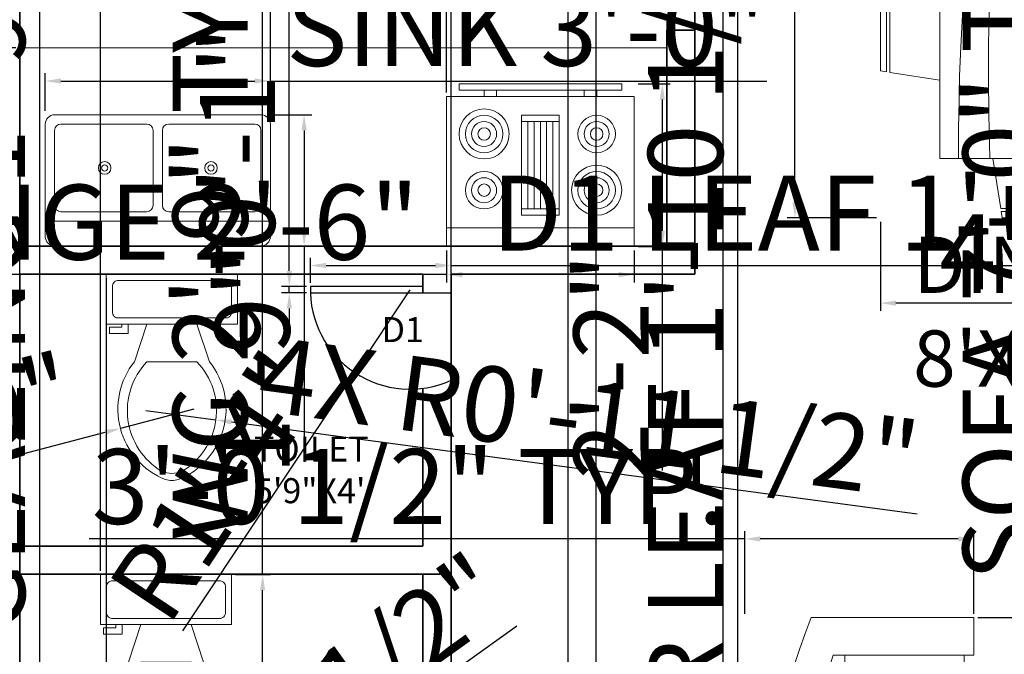
# Model space of a CAD drawing. Units: inches. Extents: x 2691 to 3133, y 1294 to 1993.
# Tile 4 of 7: x 2777 to 2935, y 1696 to 1798. Entities that reach past the tile are written whole.
import ezdxf

# ---------------------------------------------------------------- set-up
doc = ezdxf.new("R2010")
doc.units = ezdxf.units.IN
for name, color, linetype, lineweight in [('A-ANNO-DIMS', 2, 'Continuous', 18), ('A-ANNO-TEXT', 7, 'Continuous', 18), ('A-AREA-IDEN', 7, 'Continuous', 25), ('A-DOOR', 3, 'Continuous', 25), ('A-EQPM', 8, 'Continuous', 18), ('A-FLOR-FIXT', 9, 'Continuous', 18), ('A-FURN', 8, 'Continuous', 18), ('A-WALL', 7, 'Continuous', 35)]:
    doc.layers.add(name, color=color, linetype=linetype, lineweight=lineweight)
doc.styles.get("Standard").update_dxf_attribs({"font": 'arial.ttf'})
doc.dimstyles.new('ISO-25', dxfattribs={"dimtxt": 12, "dimasz": 2.5, "dimexe": 1.25, "dimexo": 0.625, "dimtad": 1, "dimdec": 1, "dimlunit": 3, "dimtxsty": 'Standard', "dimcen": 2.5, "dimadec": 0, "dimazin": 0, "dimtfac": 1, "dimtdec": 1, "dimtmove": 0, "dimatfit": 3, "dimfxl": 1, "dimarcsym": 0})

# ---------------------------------------------------------------- blocks, each defined once
blk = doc.blocks.new('Sofa - Roundback 7 ft.')
for p, q in [((-12.00002, -32.4421), (-12.00003, -6.5971)), ((11.99997, -32.4421), (11.99998, -6.5971)), ((-36.000027, -34), (-36.000027, -11.4696)), ((35.99998, -34), (35.99998, -11.4696)), ((-35.999844, -13.3819), (35.9998, -13.3819)), ((-36.000027, -32.4421), (35.99998, -32.4421))]:
    blk.add_line(p, q)
for points in [[(-36.000027, -34), (-42.000027, -34), (-42.000027, -8)], [(41.99998, -8), (41.99998, -34), (35.99998, -34)]]:
    blk.add_lwpolyline(points)
for centre, radius, start, end in [((0, -114.25), 114.25, 68.43141, 111.5686), ((-0.00001, -127.1968), 121.1968, 72.72033, 107.2797)]:
    blk.add_arc(centre, radius, start, end)
blk = doc.blocks.new('Dining Set - 36 x 72 in.')
for p, q in [((-22, 27.5), (-22.1562, 26.50042)), ((-22, 27.5), (-6, 27.5)), ((-5.8437, 26.49966), (-6, 27.5)), ((6, 27.5), (5.8438, 26.50042)), ((6, 27.5), (22, 27.5)), ((22.1563, 26.49966), (22, 27.5)), ((-22.2343, 26.00059), (-23.4847, 17.99762)), ((-22.2304, 26), (-5.7608, 26)), ((-5.8416, 26.5), (-22.1534, 26.5)), ((-4.5152, 17.99762), (-5.7655, 25.99926)), ((5.7657, 26.00059), (4.5153, 17.99762)), ((5.7696, 26), (22.2392, 26)), ((22.1584, 26.5), (5.8466, 26.5)), ((23.4848, 17.99762), (22.2345, 25.99926)), ((36, 18), (-36, 18)), ((-36, 18), (-36, -18)), ((36, -18), (36, 18)), ((-44.0006, 8.23428), (-35.9976, 9.48474)), ((44.0006, 8.23428), (35.9976, 9.48474)), ((-45.5, 8), (-44.5004, 8.15617)), ((-45.5, 8), (-45.5, -8)), ((-44.5, -8.15843), (-44.5, 8.15338)), ((-44, 8.23041), (-44, -8.23915)), ((44, 8.23041), (44, -8.23915)), ((44.5, -8.15843), (44.5, 8.15338)), ((45.5, 8), (44.5005, 8.15617)), ((45.5, 8), (45.5, -8)), ((-44.4997, -8.15631), (-45.5, -8)), ((-35.9976, -9.48476), (-43.9993, -8.2345)), ((35.9976, -9.48476), (43.9993, -8.2345)), ((44.4997, -8.15631), (45.5, -8)), ((-36, -18), (36, -18)), ((-22.2343, -26.0006), (-23.4847, -17.99762)), ((-4.5152, -17.99762), (-5.7655, -25.99928)), ((5.7657, -26.0006), (4.5153, -17.99762)), ((23.4848, -17.99762), (22.2345, -25.99928)), ((-22.2304, -26), (-5.7608, -26)), ((-22, -27.5), (-22.1562, -26.50044)), ((-5.8416, -26.5), (-22.1534, -26.5)), ((-5.8437, -26.49967), (-6, -27.5)), ((5.7696, -26), (22.2392, -26)), ((6, -27.5), (5.8438, -26.50044)), ((22.1584, -26.5), (5.8466, -26.5)), ((22.1563, -26.49967), (22, -27.5)), ((-22, -27.5), (-6, -27.5)), ((6, -27.5), (22, -27.5))]:
    blk.add_line(p, q)
for points in [[(-36, 15), (-31.1772, 14.97754), (-26.8079, 14.91406), (-22.8538, 14.81543), (-19.276, 14.6875), (-16.0362, 14.53613), (-13.0957, 14.36718), (-10.4159, 14.18652), (-7.9583, 14), (-5.6904, 13.81315), (-3.6035, 13.63021), (-1.6954, 13.45508), (0.0365, 13.29166), (1.5945, 13.14388), (2.9811, 13.01562), (4.1988, 12.9108), (5.25, 12.83333), (6.1393, 12.78613), (6.8802, 12.76823), (7.4883, 12.77767), (7.9792, 12.8125), (8.3685, 12.87077), (8.6719, 12.95052), (8.9049, 13.0498), (9.0833, 13.16666), (9.2205, 13.29899), (9.3216, 13.44401), (9.3895, 13.59879), (9.4271, 13.76041), (9.4373, 13.92594), (9.4232, 14.09245), (9.3875, 14.257), (9.3333, 14.41666), (9.2638, 14.56917), (9.1836, 14.71484), (9.0975, 14.85465), (9.0104, 14.98958), (8.9272, 15.1206), (8.8529, 15.2487), (8.7922, 15.37483), (8.75, 15.5), (8.7305, 15.62467), (8.7344, 15.74739), (8.7617, 15.86621), (8.8125, 15.97916), (8.8867, 16.08431), (8.9844, 16.17968), (9.1055, 16.26334), (9.25, 16.33333), (9.4189, 16.38802), (9.6172, 16.42708), (9.8506, 16.45052), (10.125, 16.45833), (10.4463, 16.45052), (10.8203, 16.42708), (11.2529, 16.38802), (11.75, 16.33333), (12.3184, 16.26318), (12.9694, 16.17838), (13.7151, 16.07991), (14.5677, 15.96875), (15.5395, 15.84586), (16.6426, 15.71224), (17.8893, 15.56884), (19.2917, 15.41666), (20.859, 15.25667), (22.5879, 15.08984), (24.4721, 14.91715), (26.5052, 14.73958), (28.6809, 14.5581), (30.9929, 14.3737), (33.4347, 14.18733), (36, 14)], [(-36, 10), (-28.9766, 10.14274), (-23.1725, 10.20442), (-18.4241, 10.19775), (-14.5677, 10.13541), (-11.4399, 10.03011), (-8.877, 9.89453), (-6.7154, 9.74137), (-4.7917, 9.58333), (-2.9698, 9.43082), (-1.2246, 9.28515), (0.4415, 9.14534), (2.026, 9.01041), (3.5266, 8.87939), (4.9408, 8.7513), (6.266, 8.62516), (7.5, 8.5), (8.6411, 8.37549), (9.6914, 8.2539), (10.6538, 8.13818), (11.5312, 8.03125), (12.3267, 7.93603), (13.043, 7.85547), (13.6831, 7.79248), (14.25, 7.75), (14.7471, 7.7303), (15.1797, 7.73307), (15.5537, 7.75732), (15.875, 7.80208), (16.1494, 7.86637), (16.3828, 7.94922), (16.5811, 8.04964), (16.75, 8.16666), (16.8944, 8.29915), (17.0143, 8.44531), (17.1089, 8.60319), (17.1771, 8.77083), (17.218, 8.94629), (17.2305, 9.1276), (17.2137, 9.31282), (17.1667, 9.5), (17.0895, 9.6875), (16.987, 9.875), (16.8649, 10.0625), (16.7292, 10.25), (16.5856, 10.4375), (16.4401, 10.625), (16.2985, 10.8125), (16.1667, 11), (16.05, 11.18733), (15.9518, 11.3737), (15.8752, 11.5581), (15.8229, 11.73958), (15.798, 11.91715), (15.8034, 12.08984), (15.842, 12.25667), (15.9167, 12.41666), (16.0295, 12.56836), (16.1784, 12.70833), (16.3605, 12.83268), (16.5729, 12.9375), (16.8127, 13.01888), (17.0768, 13.07291), (17.3625, 13.0957), (17.6667, 13.08333), (17.9894, 13.03312), (18.3418, 12.94726), (18.7382, 12.82918), (19.1927, 12.68229), (19.7195, 12.51001), (20.3327, 12.31575), (21.0465, 12.10294), (21.875, 11.875), (22.8357, 11.63354), (23.959, 11.37304), (25.2786, 11.08618), (26.8282, 10.76562), (28.6414, 10.40405), (30.752, 9.99414), (33.1936, 9.52856), (36, 9)], [(-36, 5.5), (-30.7157, 5.3348), (-26.069, 5.20963), (-21.9946, 5.11767), (-18.4271, 5.05208), (-15.3009, 5.00602), (-12.5508, 4.97265), (-10.1112, 4.94515), (-7.9167, 4.91666), (-5.909, 4.88167), (-4.0586, 4.83984), (-2.3429, 4.79215), (-0.7396, 4.73958), (0.7739, 4.6831), (2.22, 4.6237), (3.6213, 4.56233), (5, 4.5), (6.373, 4.43782), (7.7344, 4.3776), (9.0723, 4.32129), (10.375, 4.27083), (11.6309, 4.22819), (12.8281, 4.19531), (13.9551, 4.17415), (15, 4.16666), (15.954, 4.17448), (16.819, 4.19791), (17.6001, 4.23698), (18.3021, 4.29166), (18.9299, 4.36198), (19.4883, 4.44791), (19.9823, 4.54948), (20.4167, 4.66666), (20.7969, 4.79899), (21.1302, 4.94401), (21.4245, 5.09879), (21.6875, 5.26041), (21.9271, 5.42594), (22.1511, 5.59245), (22.3672, 5.757), (22.5834, 5.91666), (22.8065, 6.06868), (23.0404, 6.21093), (23.2879, 6.34147), (23.5521, 6.45833), (23.8358, 6.55957), (24.142, 6.64323), (24.4735, 6.70735), (24.8334, 6.75), (25.2235, 6.76969), (25.642, 6.76692), (26.0858, 6.74267), (26.5521, 6.69791), (27.0379, 6.63362), (27.5404, 6.55078), (28.0565, 6.45036), (28.5834, 6.33333), (29.1242, 6.19987), (29.7071, 6.04687), (30.3661, 5.87044), (31.1354, 5.66666), (32.0493, 5.43164), (33.142, 5.16146), (34.4475, 4.85221), (36, 4.5)], [(-36, -1), (-30.7915, -0.6591), (-26.0195, -0.38216), (-21.6519, -0.16284), (-17.6563, 0.00521), (-14.0005, 0.12833), (-10.6523, 0.21289), (-7.5796, 0.26522), (-4.75, 0.29166), (-2.134, 0.29793), (0.2878, 0.28711), (2.5317, 0.26163), (4.6146, 0.22396), (6.5529, 0.17651), (8.3633, 0.12174), (10.0623, 0.06209), (11.6667, 0), (13.1899, -0.06201), (14.6341, -0.1211), (15.9982, -0.17432), (17.2813, -0.21875), (18.4823, -0.25147), (19.6003, -0.26953), (20.6343, -0.27002), (21.5834, -0.25), (22.4481, -0.20768), (23.2357, -0.14584), (23.9549, -0.06836), (24.6146, 0.02083), (25.2235, 0.11784), (25.7904, 0.21875), (26.3241, 0.31966), (26.8334, 0.41666), (27.3265, 0.50618), (27.8099, 0.58593), (28.2894, 0.65397), (28.7709, 0.70833), (29.2601, 0.74707), (29.763, 0.76823), (30.2855, 0.76985), (30.8334, 0.75), (31.4088, 0.70784), (31.9994, 0.64713), (32.589, 0.57275), (33.1615, 0.48958), (33.7008, 0.4025), (34.1908, 0.3164), (34.6153, 0.23616), (34.9584, 0.16666), (35.2099, 0.11165), (35.3848, 0.07031), (35.504, 0.04069), (35.5886, 0.02083), (35.6594, 0.00879), (35.7377, 0.0026), (35.8442, 0.00032), (36, 0)], [(-36, -6.5), (-27.1843, -6.31267), (-20.084, -6.1263), (-14.469, -5.9419), (-10.1094, -5.76042), (-6.7752, -5.58285), (-4.2363, -5.41016), (-2.2629, -5.24333), (-0.625, -5.08334), (0.8708, -4.93099), (2.2715, -4.78646), (3.5872, -4.64974), (4.8281, -4.52084), (6.0046, -4.39974), (7.127, -4.28646), (8.2053, -4.18099), (9.25, -4.08334), (10.2705, -3.99382), (11.2734, -3.91407), (12.2647, -3.84603), (13.25, -3.79167), (14.2354, -3.75293), (15.2266, -3.73177), (16.2295, -3.73015), (17.25, -3.75), (18.2912, -3.79248), (19.3451, -3.85547), (20.4009, -3.93604), (21.4479, -4.03125), (22.4754, -4.13819), (23.4727, -4.25391), (24.4289, -4.37549), (25.3334, -4.5), (26.1785, -4.62492), (26.9694, -4.74935), (27.7145, -4.87281), (28.4219, -4.99479), (29.1, -5.11483), (29.7572, -5.23242), (30.4016, -5.34709), (31.0417, -5.45834), (31.6837, -5.56437), (32.3262, -5.65821), (32.9658, -5.73153), (33.599, -5.77604), (34.2224, -5.78345), (34.8327, -5.74545), (35.4264, -5.65373), (36, -5.5)], [(-36, -10), (-26.4022, -9.81299), (-18.4675, -9.62891), (-11.9839, -9.45069), (-6.7396, -9.28125), (-2.5226, -9.12354), (0.8789, -8.98047), (3.6769, -8.85498), (6.0833, -8.75), (8.2767, -8.66765), (10.3021, -8.60677), (12.1712, -8.56543), (13.8958, -8.54167), (15.4876, -8.53353), (16.9583, -8.53907), (18.3197, -8.55632), (19.5834, -8.58334), (20.7616, -8.61841), (21.8685, -8.66081), (22.9188, -8.71004), (23.9271, -8.76563), (24.9081, -8.82707), (25.8763, -8.89388), (26.8465, -8.96558), (27.8334, -9.04167), (28.8474, -9.12118), (29.8828, -9.20117), (30.93, -9.27824), (31.9792, -9.34896), (33.0205, -9.40991), (34.0443, -9.45768), (35.0407, -9.48885), (36, -9.5)], [(-36, -14.5), (-30.0881, -14.33513), (-25.0332, -14.21224), (-20.7312, -14.12647), (-17.0781, -14.07292), (-13.97, -14.04671), (-11.3027, -14.04297), (-8.9724, -14.05681), (-6.875, -14.08334), (-4.9224, -14.11833), (-3.0905, -14.16016), (-1.3709, -14.20785), (0.2448, -14.26042), (1.7647, -14.3169), (3.1973, -14.3763), (4.5507, -14.43767), (5.8333, -14.5), (7.0554, -14.5621), (8.235, -14.62175), (9.3922, -14.67652), (10.5469, -14.72396), (11.7192, -14.76164), (12.929, -14.78711), (14.1965, -14.79794), (15.5417, -14.79167), (16.9933, -14.76424), (18.6152, -14.70508), (20.4804, -14.60197), (22.6615, -14.44271), (25.2312, -14.21509), (28.2624, -13.9069), (31.8277, -13.50594), (36, -13)]]:
    blk.add_lwpolyline(points)
blk = doc.blocks.new('Toilet - top')
for p, q in [((9.5, -6), (9.5, -2)), ((-10, -8.5), (-8, -8.5)), ((-10, -9.5), (-10, -8.5)), ((-8, -8.5), (-8, -8)), ((-7, -8), (-7, -9.5)), ((-4, -8), (-6, -14)), ((4, -8), (6, -14)), ((-7, -9.5), (-10, -9.5)), ((4, -14), (-4, -14))]:
    blk.add_line(p, q)
blk.add_lwpolyline([(10.5, -8), (10.5, 0), (-10.5, 0), (-10.5, -8)], close=True)
for points in [[(8.5, -1), (-8.5, -1)], [(-9.5, -2), (-9.5, -6)], [(-8.5, -7), (8.5, -7)]]:
    blk.add_lwpolyline(points)
for centre, radius, start, end in [((-8.62, -1.88), 0.884, 81.8699, 188.1301), ((8.62, -1.88), 0.884, 351.8699, 98.1301), ((-8.62, -6.12), 0.884, 171.8699, 278.1301), ((8.62, -6.12), 0.884, 261.8699, 8.1301), ((3.52, -21.58), 12.17, 141.4691, 247.9714), ((4.2, -21.82), 11.33, 136.3677, 238.9468), ((-3.52, -21.58), 12.17, 292.0284, 38.5307), ((-4.2, -21.82), 11.33, 301.053, 43.6321), ((0, -27.88), 4, 245.7318, 294.2682), ((0, -29), 4, 254.8605, 285.1395)]:
    blk.add_arc(centre, radius, start, end)
blk = doc.blocks.new('Range-Oven - 30 in top')
for p, q in [((0, -3), (30, -3)), ((12, -6), (18, -6)), ((13, -20), (13, -6)), ((14, -6), (14, -20)), ((15, -20), (15, -6)), ((16, -6), (16, -20)), ((17, -20), (17, -6)), ((18, -20), (12, -20)), ((6, -24), (6, -25)), ((8, -25), (8, -24)), ((22, -25), (22, -24)), ((24, -24), (24, -25))]:
    blk.add_line(p, q)
for points in [[(0, -24), (0, 0), (30, 0), (30, -24)], [(12, -21), (12, -5), (18, -5), (18, -21)], [(2, -26), (2, -25), (28, -25), (28, -26)]]:
    blk.add_lwpolyline(points, close=True)
for centre, radius in [((6, -9), 4), ((6, -9), 3), ((24, -9), 3), ((6, -9), 2), ((24, -9), 2), ((6, -9), 1), ((24, -9), 1), ((24, -18), 4), ((6, -18), 3), ((24, -18), 3), ((6, -18), 2), ((6, -18), 1), ((24, -18), 2), ((24, -18), 1)]:
    blk.add_circle(centre, radius)
blk = doc.blocks.new('Sink-double - 36 in top')
for p, q in [((-18, -4), (18, -4)), ((-0.75, -18.5), (-0.75, -6.5)), ((0.75, -6.5), (0.75, -18.5))]:
    blk.add_line(p, q)
for points in [[(-16.5, 0), (16.5, 0)], [(-18, -19.5), (-18, -1.5)], [(18, -1.5), (18, -19.5)], [(-15.5, -5.5), (-1.75, -5.5)], [(1.75, -5.5), (15.5, -5.5)], [(-16.5, -18.5), (-16.5, -6.5)], [(16.5, -6.5), (16.5, -18.5)], [(-1.75, -19.5), (-15.5, -19.5)], [(15.5, -19.5), (1.75, -19.5)], [(16.5, -21), (-16.5, -21)]]:
    blk.add_lwpolyline(points)
for centre, radius in [((-8.5, -12.5), 1), ((-8.5, -12.5), 0.5), ((8.5, -12.5), 1), ((8.5, -12.5), 0.5)]:
    blk.add_circle(centre, radius)
for centre, radius, start, end in [((-16.5, -1.5), 1.5, 90, 180), ((16.5, -1.5), 1.5, 0, 90), ((-15.5, -6.5), 1, 90, 180), ((-1.75, -6.5), 1, 0, 90), ((1.75, -6.5), 1, 90, 180), ((15.5, -6.5), 1, 0, 90), ((-15.5, -18.5), 1, 180, 270), ((-1.75, -18.5), 1, 270, 0), ((1.75, -18.5), 1, 180, 270), ((15.5, -18.5), 1, 270, 0), ((-16.5, -19.5), 1.5, 180, 270), ((16.5, -19.5), 1.5, 270, 0)]:
    blk.add_arc(centre, radius, start, end)
blk = doc.blocks.new('DOOR-LEAF-THIN')
for p, q in [((18, 1), (0, 1)), ((0, 1), (0, 0)), ((0, 0), (22.5, 0))]:
    blk.add_line(p, q)
blk = doc.blocks.new('*D18')
at = {"layer": 'A-ANNO-DIMS', "color": 0, "lineweight": -2, "transparency": 16777216}
for p, q in [((2780.49, 1693.45), (2780.49, 1876.36)), ((2777.87, 1693.45), (2781.74, 1693.45)), ((2780.49, 1674.35), (2780.49, 1690.95)), ((2777.87, 1671.85), (2781.74, 1671.85))]:
    blk.add_line(p, q, dxfattribs=at)
at = {"layer": 'A-ANNO-DIMS', "color": 0, "transparency": 16777216}
for points in [[(2780.07, 1690.95), (2780.91, 1690.95), (2780.49, 1693.45)], [(2780.07, 1674.35), (2780.91, 1674.35), (2780.49, 1671.85)]]:
    blk.add_solid(points, dxfattribs=at)
at = {"layer": 'Defpoints', "color": 0, "transparency": 16777216}
for p in [(2777.25, 1693.45), (2780.49, 1693.45), (2777.25, 1671.85)]:
    blk.add_point(p, dxfattribs=at)
at = {"layer": 'A-ANNO-DIMS', "color": 0, "transparency": 16777216, "insert": (2773.66, 1786.16), "char_height": 12, "attachment_point": 5, "rotation": 90}
blk.add_mtext('GLAZING 1\'-9 1/2" TYP.', dxfattribs=at)
blk = doc.blocks.new('*D20')
at = {"layer": 'A-ANNO-DIMS', "color": 0, "lineweight": -2, "transparency": 16777216}
for p, q in [((2942.46, 1702.1), (2942.46, 1829.23)), ((2930.49, 1702.1), (2943.71, 1702.1)), ((2942.46, 1620.6), (2942.46, 1699.6)), ((2930.49, 1618.1), (2943.71, 1618.1))]:
    blk.add_line(p, q, dxfattribs=at)
at = {"layer": 'A-ANNO-DIMS', "color": 0, "transparency": 16777216}
for points in [[(2942.05, 1699.6), (2942.88, 1699.6), (2942.46, 1702.1)], [(2942.05, 1620.6), (2942.88, 1620.6), (2942.46, 1618.1)]]:
    blk.add_solid(points, dxfattribs=at)
at = {"layer": 'Defpoints', "color": 0, "transparency": 16777216}
for p in [(2929.86, 1702.1), (2942.46, 1702.1), (2929.86, 1618.1)]:
    blk.add_point(p, dxfattribs=at)
at = {"layer": 'A-ANNO-DIMS', "color": 0, "transparency": 16777216, "insert": (2935.63, 1766.91), "char_height": 12, "attachment_point": 5, "rotation": 90}
blk.add_mtext('SOFA 7\'-0" TYP.', dxfattribs=at)
blk = doc.blocks.new('*D21')
at = {"layer": 'A-ANNO-DIMS', "color": 0, "lineweight": -2, "transparency": 16777216}
for p, q in [((2893.2, 1702.72), (2893.2, 1715.95)), ((2929.86, 1702.72), (2929.86, 1715.95)), ((2893.2, 1714.7), (2788.35, 1714.7)), ((2927.36, 1714.7), (2895.7, 1714.7))]:
    blk.add_line(p, q, dxfattribs=at)
at = {"layer": 'A-ANNO-DIMS', "color": 0, "transparency": 16777216}
for points in [[(2895.7, 1715.11), (2895.7, 1714.28), (2893.2, 1714.7)], [(2927.36, 1715.11), (2927.36, 1714.28), (2929.86, 1714.7)]]:
    blk.add_solid(points, dxfattribs=at)
at = {"layer": 'Defpoints', "color": 0, "transparency": 16777216}
for p in [(2893.2, 1714.7), (2893.2, 1702.1), (2929.86, 1702.1)]:
    blk.add_point(p, dxfattribs=at)
at = {"layer": 'A-ANNO-DIMS', "color": 0, "transparency": 16777216, "insert": (2839.52, 1721.53), "char_height": 12, "attachment_point": 5}
blk.add_mtext('3\'-0 1/2" TYP.', dxfattribs=at)
blk = doc.blocks.new('*D22')
at = {"layer": 'A-ANNO-DIMS', "color": 0, "lineweight": -2, "transparency": 16777216}
for p, q in [((2816.11, 1708.98), (2816.11, 1818.95)), ((2811.78, 1708.98), (2817.36, 1708.98)), ((2816.11, 1678.43), (2816.11, 1706.48)), ((2811.78, 1675.93), (2817.36, 1675.93))]:
    blk.add_line(p, q, dxfattribs=at)
at = {"layer": 'A-ANNO-DIMS', "color": 0, "transparency": 16777216}
for points in [[(2815.69, 1706.48), (2816.52, 1706.48), (2816.11, 1708.98)], [(2815.69, 1678.43), (2816.52, 1678.43), (2816.11, 1675.93)]]:
    blk.add_solid(points, dxfattribs=at)
at = {"layer": 'Defpoints', "color": 0, "transparency": 16777216}
for p in [(2811.15, 1708.98), (2816.11, 1708.98), (2811.15, 1675.93)]:
    blk.add_point(p, dxfattribs=at)
at = {"layer": 'A-ANNO-DIMS', "color": 0, "transparency": 16777216, "insert": (2809.28, 1765.22), "char_height": 12, "attachment_point": 5, "rotation": 90}
blk.add_mtext('WC 2\'-9" TYP.', dxfattribs=at)
blk = doc.blocks.new('*D24')
at = {"layer": 'A-ANNO-DIMS', "color": 0, "lineweight": -2, "transparency": 16777216}
for p, q in [((2823.75, 1755.69), (2823.75, 1759.69)), ((2846.25, 1755.69), (2846.25, 1759.69)), ((2826.25, 1758.44), (2843.75, 1758.44)), ((2846.25, 1758.44), (3032.5, 1758.44))]:
    blk.add_line(p, q, dxfattribs=at)
at = {"layer": 'A-ANNO-DIMS', "color": 0, "transparency": 16777216}
for points in [[(2826.25, 1758.86), (2826.25, 1758.02), (2823.75, 1758.44)], [(2843.75, 1758.86), (2843.75, 1758.02), (2846.25, 1758.44)]]:
    blk.add_solid(points, dxfattribs=at)
at = {"layer": 'Defpoints', "color": 0, "transparency": 16777216}
for p in [(2846.25, 1758.44), (2823.75, 1755.06), (2846.25, 1755.06)]:
    blk.add_point(p, dxfattribs=at)
at = {"layer": 'A-ANNO-DIMS', "color": 0, "transparency": 16777216, "insert": (2940.63, 1765.27), "char_height": 12, "attachment_point": 5}
blk.add_mtext('D1 LEAF 1\'-10 1/2" TYP.', dxfattribs=at)
blk = doc.blocks.new('*D25')
at = {"layer": 'A-ANNO-DIMS', "color": 0, "lineweight": -2, "transparency": 16777216}
for p, q in [((2820.37, 1757.56), (2820.37, 1834.46)), ((2823.12, 1755.06), (2819.12, 1755.06)), ((2820.37, 1754.06), (2820.37, 1755.06)), ((2823.12, 1754.06), (2819.12, 1754.06)), ((2820.37, 1751.56), (2820.37, 1749.06))]:
    blk.add_line(p, q, dxfattribs=at)
at = {"layer": 'A-ANNO-DIMS', "color": 0, "transparency": 16777216}
for points in [[(2819.96, 1757.56), (2820.79, 1757.56), (2820.37, 1755.06)], [(2819.96, 1751.56), (2820.79, 1751.56), (2820.37, 1754.06)]]:
    blk.add_solid(points, dxfattribs=at)
at = {"layer": 'Defpoints', "color": 0, "transparency": 16777216}
for p in [(2820.37, 1755.06), (2823.75, 1755.06), (2823.75, 1754.06)]:
    blk.add_point(p, dxfattribs=at)
at = {"layer": 'A-ANNO-DIMS', "color": 0, "transparency": 16777216, "insert": (2813.62, 1797.26), "char_height": 12, "attachment_point": 5, "rotation": 90}
blk.add_mtext('0\'-1" TYP.', dxfattribs=at)
blk = doc.blocks.new('*D26')
at = {"layer": 'A-ANNO-DIMS', "color": 0, "lineweight": -2, "transparency": 16777216}
for p, q in [((2892.12, 1644.55), (2892.12, 1859.67)), ((2889.37, 1644.55), (2893.37, 1644.55)), ((2892.12, 1624.55), (2892.12, 1642.05)), ((2889.37, 1622.05), (2893.37, 1622.05))]:
    blk.add_line(p, q, dxfattribs=at)
at = {"layer": 'A-ANNO-DIMS', "color": 0, "transparency": 16777216}
for points in [[(2891.71, 1642.05), (2892.54, 1642.05), (2892.12, 1644.55)], [(2891.71, 1624.55), (2892.54, 1624.55), (2892.12, 1622.05)]]:
    blk.add_solid(points, dxfattribs=at)
at = {"layer": 'Defpoints', "color": 0, "transparency": 16777216}
for p in [(2888.75, 1644.55), (2892.12, 1644.55), (2888.75, 1622.05)]:
    blk.add_point(p, dxfattribs=at)
at = {"layer": 'A-ANNO-DIMS', "color": 0, "transparency": 16777216, "insert": (2885.29, 1753.36), "char_height": 12, "attachment_point": 5, "rotation": 90}
blk.add_mtext('DOOR LEAF 1\'-10 1/2" TYP.', dxfattribs=at)
blk = doc.blocks.new('*D30')
at = {"layer": 'A-ANNO-DIMS', "color": 0, "lineweight": -2, "transparency": 16777216}
for p, q in [((2901.25, 1857.07), (2901.25, 1992.71)), ((2914.28, 1857.07), (2900, 1857.07)), ((2901.25, 1768.57), (2901.25, 1854.57)), ((2914.28, 1766.07), (2900, 1766.07))]:
    blk.add_line(p, q, dxfattribs=at)
at = {"layer": 'A-ANNO-DIMS', "color": 0, "transparency": 16777216}
for points in [[(2900.84, 1854.57), (2901.67, 1854.57), (2901.25, 1857.07)], [(2900.84, 1768.57), (2901.67, 1768.57), (2901.25, 1766.07)]]:
    blk.add_solid(points, dxfattribs=at)
at = {"layer": 'Defpoints', "color": 0, "transparency": 16777216}
for p in [(2901.25, 1857.07), (2914.9, 1857.07), (2914.9, 1766.07)]:
    blk.add_point(p, dxfattribs=at)
at = {"layer": 'A-ANNO-DIMS', "color": 0, "transparency": 16777216, "insert": (2894.42, 1926.14), "char_height": 12, "attachment_point": 5, "rotation": 90}
blk.add_mtext('DINING SET 7\'-7"', dxfattribs=at)
blk = doc.blocks.new('*D31')
at = {"layer": 'A-ANNO-DIMS', "color": 0, "lineweight": -2, "transparency": 16777216}
for p, q in [((2914.9, 1765.45), (2914.9, 1751.17)), ((2969.9, 1765.45), (2969.9, 1751.17)), ((2967.4, 1752.42), (2917.4, 1752.42))]:
    blk.add_line(p, q, dxfattribs=at)
at = {"layer": 'A-ANNO-DIMS', "color": 0, "transparency": 16777216}
for points in [[(2917.4, 1752.84), (2917.4, 1752), (2914.9, 1752.42)], [(2967.4, 1752.84), (2967.4, 1752), (2969.9, 1752.42)]]:
    blk.add_solid(points, dxfattribs=at)
at = {"layer": 'Defpoints', "color": 0, "transparency": 16777216}
for p in [(2914.9, 1766.07), (2969.9, 1766.07), (2914.9, 1752.42)]:
    blk.add_point(p, dxfattribs=at)
at = {"layer": 'A-ANNO-DIMS', "color": 0, "transparency": 16777216, "insert": (2942.4, 1759.05), "char_height": 12, "attachment_point": 5}
blk.add_mtext('4\'-7"', dxfattribs=at)
blk = doc.blocks.new('*D34')
at = {"layer": 'A-ANNO-DIMS', "color": 0, "lineweight": -2, "transparency": 16777216}
for p, q in [((2845.53, 1760.85), (2845.53, 1755.73)), ((2875.53, 1760.85), (2875.53, 1755.73)), ((2845.53, 1756.98), (2746.23, 1756.98)), ((2873.03, 1756.98), (2848.03, 1756.98))]:
    blk.add_line(p, q, dxfattribs=at)
at = {"layer": 'A-ANNO-DIMS', "color": 0, "transparency": 16777216}
for points in [[(2848.03, 1757.39), (2848.03, 1756.56), (2845.53, 1756.98)], [(2873.03, 1757.39), (2873.03, 1756.56), (2875.53, 1756.98)]]:
    blk.add_solid(points, dxfattribs=at)
at = {"layer": 'Defpoints', "color": 0, "transparency": 16777216}
for p in [(2845.53, 1761.48), (2875.53, 1761.48), (2845.53, 1756.98)]:
    blk.add_point(p, dxfattribs=at)
at = {"layer": 'A-ANNO-DIMS', "color": 0, "transparency": 16777216, "insert": (2794.63, 1763.81), "char_height": 12, "attachment_point": 5}
blk.add_mtext('RANGE 2\'-6"', dxfattribs=at)
blk = doc.blocks.new('*D35')
at = {"layer": 'A-ANNO-DIMS', "color": 0, "lineweight": -2, "transparency": 16777216}
for p, q in [((2876.16, 1787.48), (2881.28, 1787.48)), ((2880.03, 1784.98), (2880.03, 1763.98)), ((2876.16, 1761.48), (2881.28, 1761.48)), ((2880.03, 1761.48), (2880.03, 1725.62))]:
    blk.add_line(p, q, dxfattribs=at)
at = {"layer": 'A-ANNO-DIMS', "color": 0, "transparency": 16777216}
for points in [[(2879.61, 1784.98), (2880.45, 1784.98), (2880.03, 1787.48)], [(2879.61, 1763.98), (2880.45, 1763.98), (2880.03, 1761.48)]]:
    blk.add_solid(points, dxfattribs=at)
at = {"layer": 'Defpoints', "color": 0, "transparency": 16777216}
for p in [(2875.53, 1787.48), (2875.53, 1761.48), (2880.03, 1761.48)]:
    blk.add_point(p, dxfattribs=at)
at = {"layer": 'A-ANNO-DIMS', "color": 0, "transparency": 16777216, "insert": (2873.38, 1742.3), "char_height": 12, "attachment_point": 5, "rotation": 90}
blk.add_mtext('2\'-2"', dxfattribs=at)
blk = doc.blocks.new('*D36')
at = {"layer": 'A-ANNO-DIMS', "color": 0, "lineweight": -2, "transparency": 16777216}
for p, q in [((2781.34, 1783.18), (2781.34, 1789.2)), ((2817.34, 1783.18), (2817.34, 1789.2)), ((2783.84, 1787.95), (2814.84, 1787.95)), ((2817.34, 1787.95), (2896.72, 1787.95))]:
    blk.add_line(p, q, dxfattribs=at)
at = {"layer": 'A-ANNO-DIMS', "color": 0, "transparency": 16777216}
for points in [[(2783.84, 1788.37), (2783.84, 1787.54), (2781.34, 1787.95)], [(2814.84, 1788.37), (2814.84, 1787.54), (2817.34, 1787.95)]]:
    blk.add_solid(points, dxfattribs=at)
at = {"layer": 'Defpoints', "color": 0, "transparency": 16777216}
for p in [(2817.34, 1787.95), (2781.34, 1782.55), (2817.34, 1782.55)]:
    blk.add_point(p, dxfattribs=at)
at = {"layer": 'A-ANNO-DIMS', "color": 0, "transparency": 16777216, "insert": (2858.28, 1794.79), "char_height": 12, "attachment_point": 5}
blk.add_mtext('SINK 3\'-0"', dxfattribs=at)
blk = doc.blocks.new('*D37')
at = {"layer": 'A-ANNO-DIMS', "color": 0, "lineweight": -2, "transparency": 16777216}
for p, q in [((2817.96, 1782.55), (2823.99, 1782.55)), ((2822.74, 1780.05), (2822.74, 1764.05)), ((2817.96, 1761.55), (2823.99, 1761.55)), ((2822.74, 1761.55), (2822.74, 1727.04))]:
    blk.add_line(p, q, dxfattribs=at)
at = {"layer": 'A-ANNO-DIMS', "color": 0, "transparency": 16777216}
for points in [[(2822.32, 1780.05), (2823.16, 1780.05), (2822.74, 1782.55)], [(2822.32, 1764.05), (2823.16, 1764.05), (2822.74, 1761.55)]]:
    blk.add_solid(points, dxfattribs=at)
at = {"layer": 'Defpoints', "color": 0, "transparency": 16777216}
for p in [(2817.34, 1782.55), (2817.34, 1761.55), (2822.74, 1761.55)]:
    blk.add_point(p, dxfattribs=at)
at = {"layer": 'A-ANNO-DIMS', "color": 0, "transparency": 16777216, "insert": (2815.99, 1743.05), "char_height": 12, "attachment_point": 5, "rotation": 90}
blk.add_mtext('1\'-9"', dxfattribs=at)
blk = doc.blocks.new('*D45')
at = {"layer": 'A-ANNO-DIMS', "color": 0, "lineweight": -2, "transparency": 16777216}
for p, q in [((2744.4, 1671.85), (2744.4, 1707.71)), ((2767.62, 1671.85), (2743.15, 1671.85)), ((2744.4, 1642.55), (2744.4, 1669.35)), ((2776.62, 1640.05), (2743.15, 1640.05))]:
    blk.add_line(p, q, dxfattribs=at)
at = {"layer": 'A-ANNO-DIMS', "color": 0, "transparency": 16777216}
for points in [[(2743.98, 1669.35), (2744.82, 1669.35), (2744.4, 1671.85)], [(2743.98, 1642.55), (2744.82, 1642.55), (2744.4, 1640.05)]]:
    blk.add_solid(points, dxfattribs=at)
at = {"layer": 'Defpoints', "color": 0, "transparency": 16777216}
for p in [(2744.4, 1671.85), (2768.25, 1671.85), (2777.25, 1640.05)]:
    blk.add_point(p, dxfattribs=at)
at = {"layer": 'A-ANNO-DIMS', "color": 0, "transparency": 16777216, "insert": (2737.65, 1691.03), "char_height": 12, "attachment_point": 5, "rotation": 90}
blk.add_mtext('2\'-8"', dxfattribs=at)
blk = doc.blocks.new('*D54')
at = {"layer": 'A-ANNO-DIMS', "color": 0, "lineweight": -2, "transparency": 16777216}
for p, q in [((2846.25, 1645.18), (2846.25, 1905.15)), ((2848.75, 1903.9), (2866.94, 1903.9)), ((2869.44, 1645.18), (2869.44, 1905.15)), ((2869.44, 1903.9), (2913.28, 1903.9))]:
    blk.add_line(p, q, dxfattribs=at)
at = {"layer": 'A-ANNO-DIMS', "color": 0, "transparency": 16777216}
for points in [[(2848.75, 1904.32), (2848.75, 1903.49), (2846.25, 1903.9)], [(2866.94, 1904.32), (2866.94, 1903.49), (2869.44, 1903.9)]]:
    blk.add_solid(points, dxfattribs=at)
at = {"layer": 'Defpoints', "color": 0, "transparency": 16777216}
for p in [(2869.44, 1903.9), (2846.25, 1644.55), (2869.44, 1644.55)]:
    blk.add_point(p, dxfattribs=at)
at = {"layer": 'A-ANNO-DIMS', "color": 0, "transparency": 16777216, "insert": (2892.61, 1910.55), "char_height": 12, "attachment_point": 5}
blk.add_mtext('1\'-11"', dxfattribs=at)
blk = doc.blocks.new('*D57')
at = {"layer": 'A-ANNO-DIMS', "color": 0, "lineweight": -2, "transparency": 16777216}
for p, q in [((2777.25, 1709.68), (2777.25, 1905.15)), ((2779.75, 1903.9), (2787.65, 1903.9)), ((2790.15, 1709.61), (2790.15, 1905.15)), ((2790.15, 1903.9), (2824.67, 1903.9))]:
    blk.add_line(p, q, dxfattribs=at)
at = {"layer": 'A-ANNO-DIMS', "color": 0, "transparency": 16777216}
for points in [[(2779.75, 1904.32), (2779.75, 1903.49), (2777.25, 1903.9)], [(2787.65, 1904.32), (2787.65, 1903.49), (2790.15, 1903.9)]]:
    blk.add_solid(points, dxfattribs=at)
at = {"layer": 'Defpoints', "color": 0, "transparency": 16777216}
for p in [(2790.15, 1903.9), (2777.25, 1709.05), (2790.15, 1708.98)]:
    blk.add_point(p, dxfattribs=at)
at = {"layer": 'A-ANNO-DIMS', "color": 0, "transparency": 16777216, "insert": (2808.66, 1910.55), "char_height": 12, "attachment_point": 5}
blk.add_mtext('1\'-1"', dxfattribs=at)
blk = doc.blocks.new('*D58')
at = {"layer": 'A-ANNO-DIMS', "color": 0, "lineweight": -2, "transparency": 16777216}
for p, q in [((2777.25, 1756.43), (2777.25, 1398.95)), ((2791.1, 1756.43), (2791.1, 1398.95)), ((2779.75, 1400.2), (2788.6, 1400.2)), ((2791.1, 1400.2), (2825.62, 1400.2))]:
    blk.add_line(p, q, dxfattribs=at)
at = {"layer": 'A-ANNO-DIMS', "color": 0, "transparency": 16777216}
for points in [[(2779.75, 1400.62), (2779.75, 1399.79), (2777.25, 1400.2)], [(2788.6, 1400.62), (2788.6, 1399.79), (2791.1, 1400.2)]]:
    blk.add_solid(points, dxfattribs=at)
at = {"layer": 'Defpoints', "color": 0, "transparency": 16777216}
for p in [(2777.25, 1757.05), (2791.1, 1757.05), (2791.1, 1400.2)]:
    blk.add_point(p, dxfattribs=at)
at = {"layer": 'A-ANNO-DIMS', "color": 0, "transparency": 16777216, "insert": (2809.61, 1406.85), "char_height": 12, "attachment_point": 5}
blk.add_mtext('1\'-2"', dxfattribs=at)
blk = doc.blocks.new('*D59')
at = {"layer": 'A-ANNO-DIMS', "color": 0, "lineweight": -2, "transparency": 16777216}
for p, q in [((2776.62, 1793.25), (2743.15, 1793.25)), ((2744.4, 1790.75), (2744.4, 1764.05)), ((2776.62, 1761.55), (2743.15, 1761.55)), ((2744.4, 1761.55), (2744.4, 1697.74))]:
    blk.add_line(p, q, dxfattribs=at)
at = {"layer": 'A-ANNO-DIMS', "color": 0, "transparency": 16777216}
for points in [[(2743.98, 1790.75), (2744.82, 1790.75), (2744.4, 1793.25)], [(2743.98, 1764.05), (2744.82, 1764.05), (2744.4, 1761.55)]]:
    blk.add_solid(points, dxfattribs=at)
at = {"layer": 'Defpoints', "color": 0, "transparency": 16777216}
for p in [(2777.25, 1793.25), (2744.4, 1761.55), (2777.25, 1761.55)]:
    blk.add_point(p, dxfattribs=at)
at = {"layer": 'A-ANNO-DIMS', "color": 0, "transparency": 16777216, "insert": (2737.57, 1728.4), "char_height": 12, "attachment_point": 5, "rotation": 90}
blk.add_mtext('2\'-7 1/2"', dxfattribs=at)
blk = doc.blocks.new('*D60')
at = {"layer": 'A-ANNO-DIMS', "color": 0, "lineweight": -2, "transparency": 16777216}
for p, q in [((2817.34, 1781.68), (2817.34, 1905.15)), ((2819.84, 1903.9), (2843.03, 1903.9)), ((2845.53, 1786.1), (2845.53, 1905.15)), ((2845.53, 1903.9), (2881.38, 1903.9))]:
    blk.add_line(p, q, dxfattribs=at)
at = {"layer": 'A-ANNO-DIMS', "color": 0, "transparency": 16777216}
for points in [[(2819.84, 1904.32), (2819.84, 1903.49), (2817.34, 1903.9)], [(2843.03, 1904.32), (2843.03, 1903.49), (2845.53, 1903.9)]]:
    blk.add_solid(points, dxfattribs=at)
at = {"layer": 'Defpoints', "color": 0, "transparency": 16777216}
for p in [(2845.53, 1903.9), (2845.53, 1785.48), (2817.34, 1781.05)]:
    blk.add_point(p, dxfattribs=at)
at = {"layer": 'A-ANNO-DIMS', "color": 0, "transparency": 16777216, "insert": (2864.71, 1910.55), "char_height": 12, "attachment_point": 5}
blk.add_mtext('2\'-4"', dxfattribs=at)
blk = doc.blocks.new('*D61')
at = {"layer": 'A-ANNO-DIMS', "color": 0, "lineweight": -2, "transparency": 16777216}
for p, q in [((2864.96, 1433.88), (2864.96, 1905.15)), ((2867.46, 1903.9), (2887.25, 1903.9)), ((2889.75, 1433.68), (2889.75, 1905.15)), ((2889.75, 1903.9), (2925.6, 1903.9))]:
    blk.add_line(p, q, dxfattribs=at)
at = {"layer": 'A-ANNO-DIMS', "color": 0, "transparency": 16777216}
for points in [[(2867.46, 1904.32), (2867.46, 1903.49), (2864.96, 1903.9)], [(2887.25, 1904.32), (2887.25, 1903.49), (2889.75, 1903.9)]]:
    blk.add_solid(points, dxfattribs=at)
at = {"layer": 'Defpoints', "color": 0, "transparency": 16777216}
for p in [(2889.75, 1903.9), (2864.96, 1433.26), (2889.75, 1433.05)]:
    blk.add_point(p, dxfattribs=at)
at = {"layer": 'A-ANNO-DIMS', "color": 0, "transparency": 16777216, "insert": (2908.93, 1910.55), "char_height": 12, "attachment_point": 5}
blk.add_mtext('2\'-1"', dxfattribs=at)
blk = doc.blocks.new('*D64')
at = {"layer": 'A-ANNO-DIMS', "color": 0, "lineweight": -2, "transparency": 16777216}
for p, q in [((2856.77, 1700.76), (2795.71, 1657.05)), ((2780.12, 1645.9), (2793.67, 1655.6))]:
    blk.add_line(p, q, dxfattribs=at)
at = {"layer": 'A-ANNO-DIMS', "color": 0, "transparency": 16777216}
blk.add_solid([(2795.46, 1657.39), (2795.95, 1656.71), (2793.67, 1655.6)], dxfattribs=at)
at = {"layer": 'Defpoints', "color": 0, "transparency": 16777216}
for p in [(2793.67, 1655.6), (2780.12, 1645.9)]:
    blk.add_point(p, dxfattribs=at)
at = {"layer": 'A-ANNO-DIMS', "color": 0, "transparency": 16777216, "insert": (2823.28, 1685.19), "char_height": 12, "attachment_point": 5, "rotation": 35.5904}
blk.add_mtext('R1\'-4 1/2"', dxfattribs=at)
blk = doc.blocks.new('*D65')
at = {"layer": 'A-ANNO-DIMS', "color": 0, "lineweight": -2, "transparency": 16777216}
for p, q in [((2839.65, 1754.56), (2830.84, 1741.32)), ((2803.33, 1700), (2829.45, 1739.24))]:
    blk.add_line(p, q, dxfattribs=at)
at = {"layer": 'A-ANNO-DIMS', "color": 0, "transparency": 16777216}
blk.add_solid([(2829.1, 1739.47), (2829.8, 1739.01), (2830.84, 1741.32)], dxfattribs=at)
at = {"layer": 'Defpoints', "color": 0, "transparency": 16777216}
for p in [(2839.65, 1754.56), (2830.84, 1741.32)]:
    blk.add_point(p, dxfattribs=at)
at = {"layer": 'A-ANNO-DIMS', "color": 0, "transparency": 16777216, "insert": (2810.16, 1722.27), "char_height": 12, "attachment_point": 5, "rotation": 56.3517}
blk.add_mtext('R1\'-4"', dxfattribs=at)
blk = doc.blocks.new('*D68')
at = {"layer": 'A-ANNO-DIMS', "color": 0, "lineweight": -2, "transparency": 16777216}
for p, q in [((2805.12, 1735.47), (2793.35, 1732.38)), ((2719.94, 1713.09), (2790.93, 1731.75))]:
    blk.add_line(p, q, dxfattribs=at)
at = {"layer": 'A-ANNO-DIMS', "color": 0, "transparency": 16777216}
blk.add_solid([(2790.82, 1732.15), (2791.03, 1731.34), (2793.35, 1732.38)], dxfattribs=at)
at = {"layer": 'Defpoints', "color": 0, "transparency": 16777216}
for p in [(2805.12, 1735.47), (2793.35, 1732.38)]:
    blk.add_point(p, dxfattribs=at)
at = {"layer": 'A-ANNO-DIMS', "color": 0, "transparency": 16777216, "insert": (2752.51, 1728.63), "char_height": 12, "attachment_point": 5, "rotation": 14.721}
blk.add_mtext('4X R1\'-0"', dxfattribs=at)
blk = doc.blocks.new('*D69')
at = {"layer": 'A-ANNO-DIMS', "color": 0, "lineweight": -2, "transparency": 16777216}
for p, q in [((2797.4, 1735.24), (2808.62, 1733.73)), ((2920.8, 1718.65), (2811.1, 1733.39))]:
    blk.add_line(p, q, dxfattribs=at)
at = {"layer": 'A-ANNO-DIMS', "color": 0, "transparency": 16777216}
blk.add_solid([(2811.16, 1733.81), (2811.05, 1732.98), (2808.62, 1733.73)], dxfattribs=at)
at = {"layer": 'Defpoints', "color": 0, "transparency": 16777216}
for p in [(2797.4, 1735.24), (2808.62, 1733.73)]:
    blk.add_point(p, dxfattribs=at)
at = {"layer": 'A-ANNO-DIMS', "color": 0, "transparency": 16777216, "insert": (2868.1, 1732.62), "char_height": 12, "attachment_point": 5, "rotation": 352.343}
blk.add_mtext('4X R0\'-11 1/2"', dxfattribs=at)

msp = doc.modelspace()

# ---------------------------------------------------------------- linework, layer by layer
at = {"layer": 'A-DOOR'}
msp.add_arc((2839.65, 1754.56), 15.91, 178.199, 294.5047, dxfattribs=at)
at = {"layer": 'A-FLOR-FIXT'}
msp.add_line((2880.75, 1793.25), (2777.25, 1793.25), dxfattribs=at)
at = {"layer": 'A-WALL'}
for p, q in [((2777.25, 1871.05), (2777.25, 1761.55)), ((2885.25, 1796.11), (2885.25, 1871.05)), ((2880.75, 1796.11), (2880.75, 1761.55)), ((2880.75, 1796.11), (2885.25, 1796.11)), ((2885.25, 1796.11), (2885.25, 1757.05)), ((2880.75, 1761.55), (2777.25, 1761.55)), ((2777.25, 1757.05), (2777.25, 1644.55)), ((2841.75, 1757.05), (2777.25, 1757.05)), ((2841.75, 1757.05), (2841.75, 1755.06)), ((2841.75, 1757.05), (2841.75, 1754.06)), ((2885.25, 1757.05), (2846.25, 1757.05)), ((2846.25, 1757.05), (2846.25, 1709.05)), ((2846.25, 1757.05), (2846.25, 1644.55)), ((2846.25, 1754.06), (2846.25, 1740.09)), ((2841.75, 1738.79), (2841.75, 1713.55)), ((2841.75, 1738.79), (2841.75, 1713.55)), ((2841.75, 1713.55), (2777.25, 1713.55)), ((2846.25, 1709.05), (2777.25, 1709.05)), ((2841.75, 1709.05), (2841.75, 1644.55))]:
    msp.add_line(p, q, dxfattribs=at)

# ---------------------------------------------------------------- block references
at = {"layer": 'A-DOOR'}
msp.add_blockref('DOOR-LEAF-THIN', (2823.75, 1754.06), dxfattribs=at)
at = {"layer": 'A-EQPM', "rotation": 180}
msp.add_blockref('Range-Oven - 30 in top', (2875.53, 1761.48), dxfattribs=at)
at = {"layer": 'A-FLOR-FIXT', "xscale": -1, "rotation": 180}
msp.add_blockref('Sink-double - 36 in top', (2799.34, 1761.55), dxfattribs=at)
at = {"layer": 'A-FLOR-FIXT'}
for p in [(2801.6, 1757.05), (2800.65, 1708.98)]:
    msp.add_blockref('Toilet - top', p, dxfattribs=at)
at = {"layer": 'A-FURN', "rotation": 90}
for name, p in [('Dining Set - 36 x 72 in.', (2942.4, 1811.57)), ('Sofa - Roundback 7 ft.', (2895.86, 1660.1))]:
    msp.add_blockref(name, p, dxfattribs=at)

# ---------------------------------------------------------------- texts
at = {"layer": 'A-ANNO-TEXT', "insert": (2835.12, 1750.18), "char_height": 4, "attachment_point": 1}
msp.add_mtext_dynamic_manual_height_columns('D1', width=0.1038, gutter_width=12.5, heights=[0], dxfattribs=at)
at = {"layer": 'A-AREA-IDEN', "insert": (2920.14, 1763.05), "char_height": 9, "attachment_point": 1}
msp.add_mtext("DINING \\P8'X10'", dxfattribs=at)
at = {"layer": 'A-AREA-IDEN', "insert": (2814.72, 1731.08), "char_height": 4, "attachment_point": 1}
msp.add_mtext_dynamic_manual_height_columns('TOILET\\P5\'9"X4\'', width=1.3496, gutter_width=12.5, heights=[0], dxfattribs=at)

# ---------------------------------------------------------------- dimensions: what is measured, and where the dimension line sits
at = {"layer": 'A-ANNO-DIMS'}
for base, p1, p2, angle, text, picture, middle in [((2901.25, 1857.07), (2914.9, 1766.07), (2914.9, 1857.07), 90, 'DINING SET <>', '*D30', (2894.42, 1926.14)), ((2780.49, 1693.45), (2777.25, 1671.85), (2777.25, 1693.45), 90, 'GLAZING <> TYP.', '*D18', (2773.66, 1786.16)), ((2892.12, 1644.55), (2888.75, 1622.05), (2888.75, 1644.55), 90, 'DOOR LEAF <> TYP.', '*D26', (2885.29, 1753.36)), ((2820.37, 1755.06), (2823.75, 1754.06), (2823.75, 1755.06), 90, '<> TYP.', '*D25', (2813.62, 1797.26)), ((2942.46, 1702.1), (2929.86, 1618.1), (2929.86, 1702.1), 90, 'SOFA <> TYP.', '*D20', (2935.63, 1766.91)), ((2816.1072, 1708.9801), (2811.1502, 1675.9339), (2811.1502, 1708.9801), 90, 'WC <> TYP.', '*D22', (2809.2775, 1765.217)), ((2845.53, 1756.98), (2875.53, 1761.48), (2845.53, 1761.48), 180, 'RANGE <>', '*D34', (2794.63, 1763.81)), ((2893.2, 1714.7), (2929.86, 1702.1), (2893.2, 1702.1), 180, '<> TYP.', '*D21', (2839.52, 1721.53))]:
    dim = msp.add_linear_dim(base=base, p1=p1, p2=p2, angle=angle, text=text, dimstyle='ISO-25', override={"dimdec": 1, "dimlfac": 1, "dimrnd": 0, "dimzin": 1, "dimdsep": 46, "dimlunit": 4, "dimfrac": 2}, dxfattribs=at)
    dim.commit()
    dim.dimension.update_dxf_attribs({"geometry": picture, "text_midpoint": middle})
for base, p1, p2, picture, middle in [((2790.15, 1903.9), (2777.25, 1709.05), (2790.15, 1708.98), '*D57', (2808.66, 1910.55)), ((2845.53, 1903.9), (2817.34, 1781.05), (2845.53, 1785.48), '*D60', (2864.71, 1910.55)), ((2869.44, 1903.9), (2846.25, 1644.55), (2869.44, 1644.55), '*D54', (2892.61, 1910.55)), ((2889.75, 1903.9), (2864.96, 1433.26), (2889.75, 1433.05), '*D61', (2908.93, 1910.55)), ((2791.0965, 1400.2049), (2777.2496, 1757.0549), (2791.0965, 1757.0549), '*D58', (2809.6063, 1406.8545))]:
    dim = msp.add_linear_dim(base=base, p1=p1, p2=p2, dimstyle='ISO-25', override={"dimdec": 1, "dimlfac": 1, "dimrnd": 0, "dimzin": 1, "dimdsep": 46, "dimlunit": 4, "dimfrac": 2}, dxfattribs=at)
    dim.commit()
    dim.dimension.update_dxf_attribs({"geometry": picture, "text_midpoint": middle})
for base, p1, p2, text, picture, middle in [((2817.34, 1787.95), (2781.34, 1782.55), (2817.34, 1782.55), 'SINK <>', '*D36', (2858.28, 1794.79)), ((2846.25, 1758.44), (2823.75, 1755.06), (2846.25, 1755.06), 'D1 LEAF <> TYP.', '*D24', (2940.63, 1765.27))]:
    dim = msp.add_linear_dim(base=base, p1=p1, p2=p2, text=text, dimstyle='ISO-25', override={"dimdec": 1, "dimlfac": 1, "dimrnd": 0, "dimzin": 1, "dimdsep": 46, "dimlunit": 4, "dimfrac": 2}, dxfattribs=at)
    dim.commit()
    dim.dimension.update_dxf_attribs({"geometry": picture, "text_midpoint": middle})
for base, p1, p2, angle, picture, middle in [((2744.4, 1761.55), (2777.25, 1793.25), (2777.25, 1761.55), 90, '*D59', (2737.57, 1728.4)), ((2880.03, 1761.48), (2875.53, 1787.48), (2875.53, 1761.48), 270, '*D35', (2873.38, 1742.3)), ((2822.74, 1761.55), (2817.34, 1782.55), (2817.34, 1761.55), 270, '*D37', (2815.99, 1743.05)), ((2914.9, 1752.42), (2969.9, 1766.07), (2914.9, 1766.07), 180, '*D31', (2942.4, 1759.05)), ((2744.4, 1671.85), (2777.25, 1640.05), (2768.25, 1671.85), 90, '*D45', (2737.65, 1691.03))]:
    dim = msp.add_linear_dim(base=base, p1=p1, p2=p2, angle=angle, dimstyle='ISO-25', override={"dimdec": 1, "dimlfac": 1, "dimrnd": 0, "dimzin": 1, "dimdsep": 46, "dimlunit": 4, "dimfrac": 2}, dxfattribs=at)
    dim.commit()
    dim.dimension.update_dxf_attribs({"geometry": picture, "text_midpoint": middle})
for center, mpoint, picture, middle in [((2797.4, 1735.24), (2808.62, 1733.73), '*D69', (2868.1, 1732.62)), ((2805.12, 1735.47), (2793.35, 1732.38), '*D68', (2752.51, 1728.63))]:
    dim = msp.add_radius_dim(center=center, mpoint=mpoint, text='4X <>', dimstyle='ISO-25', override={"dimdec": 1, "dimlfac": 1, "dimrnd": 0, "dimzin": 1, "dimdsep": 46, "dimlunit": 4, "dimfrac": 2}, dxfattribs=at)
    dim.commit()
    dim.dimension.update_dxf_attribs({"geometry": picture, "text_midpoint": middle})
for center, mpoint, picture, middle in [((2839.65, 1754.56), (2830.84, 1741.32), '*D65', (2810.16, 1722.27)), ((2780.12, 1645.9), (2793.67, 1655.6), '*D64', (2823.28, 1685.19))]:
    dim = msp.add_radius_dim(center=center, mpoint=mpoint, dimstyle='ISO-25', override={"dimdec": 1, "dimlfac": 1, "dimrnd": 0, "dimzin": 1, "dimdsep": 46, "dimlunit": 4, "dimfrac": 2}, dxfattribs=at)
    dim.commit()
    dim.dimension.update_dxf_attribs({"geometry": picture, "text_midpoint": middle})

doc.saveas('drawing.dxf')
